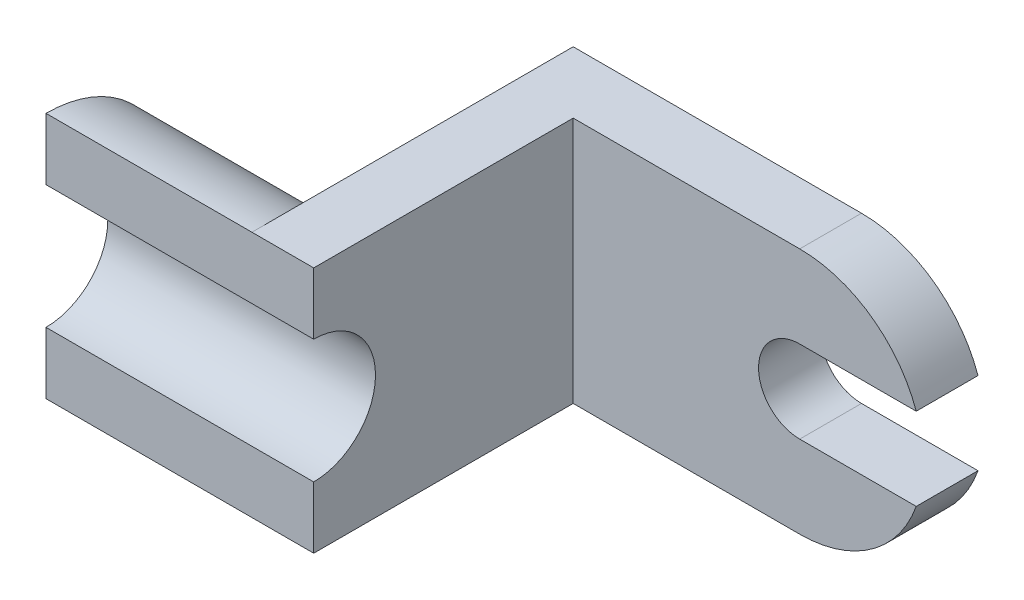
ISO-10303-21;
HEADER;
FILE_DESCRIPTION(('STEP AP214'),'2;1');
FILE_NAME('part.step','',(''),(''),'','','');
FILE_SCHEMA(('AUTOMOTIVE_DESIGN { 1 0 10303 214 1 1 1 1 }'));
ENDSEC;
DATA;
#1=APPLICATION_CONTEXT('core data for automotive mechanical design processes');
#2=APPLICATION_PROTOCOL_DEFINITION('international standard','automotive_design',2000,#1);
#3=PRODUCT_CONTEXT('',#1,'mechanical');
#4=PRODUCT('Part','Part','',(#3));
#5=PRODUCT_RELATED_PRODUCT_CATEGORY('part','',(#4));
#6=PRODUCT_DEFINITION_FORMATION('','',#4);
#7=PRODUCT_DEFINITION_CONTEXT('part definition',#1,'design');
#8=PRODUCT_DEFINITION('design','',#6,#7);
#9=PRODUCT_DEFINITION_SHAPE('','',#8);
#10=(LENGTH_UNIT() NAMED_UNIT(*) SI_UNIT(.MILLI.,.METRE.));
#11=(NAMED_UNIT(*) PLANE_ANGLE_UNIT() SI_UNIT($,.RADIAN.));
#12=(NAMED_UNIT(*) SI_UNIT($,.STERADIAN.) SOLID_ANGLE_UNIT());
#13=UNCERTAINTY_MEASURE_WITH_UNIT(LENGTH_MEASURE(1.E-05),#10,'distance_accuracy_value','');
#14=(GEOMETRIC_REPRESENTATION_CONTEXT(3) GLOBAL_UNCERTAINTY_ASSIGNED_CONTEXT((#13)) GLOBAL_UNIT_ASSIGNED_CONTEXT((#10,
#11,#12)) REPRESENTATION_CONTEXT('',''));
#15=CARTESIAN_POINT('',(0.,0.,0.));
#16=DIRECTION('',(0.,0.,1.));
#17=DIRECTION('',(1.,0.,0.));
#18=AXIS2_PLACEMENT_3D('',#15,#16,#17);
#19=CARTESIAN_POINT('',(15.,60.,78.));
#20=DIRECTION('',(0.,0.,1.));
#21=DIRECTION('',(0.,-1.,0.));
#22=AXIS2_PLACEMENT_3D('',#19,#20,#21);
#23=PLANE('',#22);
#24=DIRECTION('',(0.,1.,0.));
#25=VECTOR('',#24,1.);
#26=CARTESIAN_POINT('',(15.,60.,78.));
#27=LINE('',#26,#25);
#28=CARTESIAN_POINT('',(15.,0.,78.));
#29=VERTEX_POINT('',#28);
#30=CARTESIAN_POINT('',(15.,15.,78.));
#31=VERTEX_POINT('',#30);
#32=EDGE_CURVE('E149',#29,#31,#27,.T.);
#33=ORIENTED_EDGE('',*,*,#32,.T.);
#34=DIRECTION('',(1.,0.,0.));
#35=VECTOR('',#34,1.);
#36=CARTESIAN_POINT('',(-50.,15.,78.));
#37=LINE('',#36,#35);
#38=CARTESIAN_POINT('',(-50.,15.,78.));
#39=VERTEX_POINT('',#38);
#40=EDGE_CURVE('E132',#39,#31,#37,.T.);
#41=ORIENTED_EDGE('',*,*,#40,.F.);
#42=DIRECTION('',(0.,1.,0.));
#43=VECTOR('',#42,1.);
#44=CARTESIAN_POINT('',(-50.,15.,78.));
#45=LINE('',#44,#43);
#46=CARTESIAN_POINT('',(-50.,0.,78.));
#47=VERTEX_POINT('',#46);
#48=EDGE_CURVE('E243',#47,#39,#45,.T.);
#49=ORIENTED_EDGE('',*,*,#48,.F.);
#50=DIRECTION('',(1.,0.,0.));
#51=VECTOR('',#50,1.);
#52=CARTESIAN_POINT('',(-50.,0.,78.));
#53=LINE('',#52,#51);
#54=CARTESIAN_POINT('',(0.,0.,78.));
#55=VERTEX_POINT('',#54);
#56=EDGE_CURVE('E141',#47,#55,#53,.T.);
#57=ORIENTED_EDGE('',*,*,#56,.T.);
#58=DIRECTION('',(-1.,0.,0.));
#59=VECTOR('',#58,1.);
#60=CARTESIAN_POINT('',(15.,0.,78.));
#61=LINE('',#60,#59);
#62=EDGE_CURVE('E160',#29,#55,#61,.T.);
#63=ORIENTED_EDGE('',*,*,#62,.F.);
#64=EDGE_LOOP('',(#33,#41,#49,#57,#63));
#65=FACE_BOUND('',#64,.T.);
#66=ADVANCED_FACE('F39',(#65),#23,.T.);
#67=CARTESIAN_POINT('',(0.,0.,15.));
#68=DIRECTION('',(1.,0.,0.));
#69=DIRECTION('',(0.,0.,-1.));
#70=AXIS2_PLACEMENT_3D('',#67,#68,#69);
#71=PLANE('',#70);
#72=CARTESIAN_POINT('',(0.,30.,78.));
#73=DIRECTION('',(-1.,0.,0.));
#74=DIRECTION('',(0.,0.,1.));
#75=AXIS2_PLACEMENT_3D('',#72,#73,#74);
#76=CIRCLE('',#75,30.);
#77=CARTESIAN_POINT('',(0.,60.,78.));
#78=VERTEX_POINT('',#77);
#79=EDGE_CURVE('E155',#78,#55,#76,.T.);
#80=ORIENTED_EDGE('',*,*,#79,.F.);
#81=DIRECTION('',(0.,0.,-1.));
#82=VECTOR('',#81,1.);
#83=CARTESIAN_POINT('',(0.,60.,15.));
#84=LINE('',#83,#82);
#85=CARTESIAN_POINT('',(0.,60.,0.));
#86=VERTEX_POINT('',#85);
#87=EDGE_CURVE('E220',#78,#86,#84,.T.);
#88=ORIENTED_EDGE('',*,*,#87,.T.);
#89=DIRECTION('',(0.,-1.,0.));
#90=VECTOR('',#89,1.);
#91=CARTESIAN_POINT('',(0.,0.,0.));
#92=LINE('',#91,#90);
#93=CARTESIAN_POINT('',(0.,0.,0.));
#94=VERTEX_POINT('',#93);
#95=EDGE_CURVE('E199',#86,#94,#92,.T.);
#96=ORIENTED_EDGE('',*,*,#95,.T.);
#97=DIRECTION('',(0.,0.,-1.));
#98=VECTOR('',#97,1.);
#99=CARTESIAN_POINT('',(0.,0.,15.));
#100=LINE('',#99,#98);
#101=EDGE_CURVE('E206',#55,#94,#100,.T.);
#102=ORIENTED_EDGE('',*,*,#101,.F.);
#103=EDGE_LOOP('',(#80,#88,#96,#102));
#104=FACE_BOUND('',#103,.T.);
#105=ADVANCED_FACE('F237',(#104),#71,.F.);
#106=CARTESIAN_POINT('',(70.,30.,15.));
#107=DIRECTION('',(0.,0.,-1.));
#108=DIRECTION('',(-1.,0.,0.));
#109=AXIS2_PLACEMENT_3D('',#106,#107,#108);
#110=CYLINDRICAL_SURFACE('',#109,30.);
#111=DIRECTION('',(0.,0.,1.));
#112=VECTOR('',#111,1.);
#113=CARTESIAN_POINT('',(98.2842712474619,40.,0.));
#114=LINE('',#113,#112);
#115=CARTESIAN_POINT('',(98.2842712474619,40.,0.));
#116=VERTEX_POINT('',#115);
#117=CARTESIAN_POINT('',(98.2842712474619,40.,15.));
#118=VERTEX_POINT('',#117);
#119=EDGE_CURVE('E191',#116,#118,#114,.T.);
#120=ORIENTED_EDGE('',*,*,#119,.F.);
#121=CARTESIAN_POINT('',(70.,30.,0.));
#122=DIRECTION('',(0.,0.,1.));
#123=DIRECTION('',(-1.,0.,0.));
#124=AXIS2_PLACEMENT_3D('',#121,#122,#123);
#125=CIRCLE('',#124,30.);
#126=CARTESIAN_POINT('',(70.,60.,0.));
#127=VERTEX_POINT('',#126);
#128=EDGE_CURVE('E208',#116,#127,#125,.T.);
#129=ORIENTED_EDGE('',*,*,#128,.T.);
#130=DIRECTION('',(0.,0.,-1.));
#131=VECTOR('',#130,1.);
#132=CARTESIAN_POINT('',(70.,60.,15.));
#133=LINE('',#132,#131);
#134=CARTESIAN_POINT('',(70.,60.,15.));
#135=VERTEX_POINT('',#134);
#136=EDGE_CURVE('E50',#135,#127,#133,.T.);
#137=ORIENTED_EDGE('',*,*,#136,.F.);
#138=CARTESIAN_POINT('',(70.,30.,15.));
#139=DIRECTION('',(0.,0.,1.));
#140=DIRECTION('',(-1.,0.,0.));
#141=AXIS2_PLACEMENT_3D('',#138,#139,#140);
#142=CIRCLE('',#141,30.);
#143=EDGE_CURVE('E200',#118,#135,#142,.T.);
#144=ORIENTED_EDGE('',*,*,#143,.F.);
#145=EDGE_LOOP('',(#120,#129,#137,#144));
#146=FACE_BOUND('',#145,.T.);
#147=ADVANCED_FACE('F273',(#146),#110,.T.);
#148=CARTESIAN_POINT('',(70.,30.,15.));
#149=DIRECTION('',(0.,0.,-1.));
#150=DIRECTION('',(-1.,0.,0.));
#151=AXIS2_PLACEMENT_3D('',#148,#149,#150);
#152=PLANE('',#151);
#153=DIRECTION('',(-1.,0.,0.));
#154=VECTOR('',#153,1.);
#155=CARTESIAN_POINT('',(0.,60.,15.));
#156=LINE('',#155,#154);
#157=CARTESIAN_POINT('',(15.,60.,15.));
#158=VERTEX_POINT('',#157);
#159=EDGE_CURVE('E204',#135,#158,#156,.T.);
#160=ORIENTED_EDGE('',*,*,#159,.T.);
#161=DIRECTION('',(0.,-1.,0.));
#162=VECTOR('',#161,1.);
#163=CARTESIAN_POINT('',(15.,30.,15.));
#164=LINE('',#163,#162);
#165=CARTESIAN_POINT('',(15.,0.,15.));
#166=VERTEX_POINT('',#165);
#167=EDGE_CURVE('E65',#158,#166,#164,.T.);
#168=ORIENTED_EDGE('',*,*,#167,.T.);
#169=DIRECTION('',(1.,0.,0.));
#170=VECTOR('',#169,1.);
#171=CARTESIAN_POINT('',(70.,0.,15.));
#172=LINE('',#171,#170);
#173=CARTESIAN_POINT('',(70.,0.,15.));
#174=VERTEX_POINT('',#173);
#175=EDGE_CURVE('E197',#166,#174,#172,.T.);
#176=ORIENTED_EDGE('',*,*,#175,.T.);
#177=CARTESIAN_POINT('',(98.2842712474619,20.,15.));
#178=VERTEX_POINT('',#177);
#179=EDGE_CURVE('E203',#174,#178,#142,.T.);
#180=ORIENTED_EDGE('',*,*,#179,.T.);
#181=DIRECTION('',(1.,0.,0.));
#182=VECTOR('',#181,1.);
#183=CARTESIAN_POINT('',(0.,20.,15.));
#184=LINE('',#183,#182);
#185=CARTESIAN_POINT('',(70.,20.,15.));
#186=VERTEX_POINT('',#185);
#187=EDGE_CURVE('E184',#186,#178,#184,.T.);
#188=ORIENTED_EDGE('',*,*,#187,.F.);
#189=CARTESIAN_POINT('',(70.,30.,15.));
#190=DIRECTION('',(0.,0.,1.));
#191=DIRECTION('',(1.,0.,0.));
#192=AXIS2_PLACEMENT_3D('',#189,#190,#191);
#193=CIRCLE('',#192,9.99999999999999);
#194=CARTESIAN_POINT('',(70.,40.,15.));
#195=VERTEX_POINT('',#194);
#196=EDGE_CURVE('E173',#195,#186,#193,.T.);
#197=ORIENTED_EDGE('',*,*,#196,.F.);
#198=DIRECTION('',(1.,0.,0.));
#199=VECTOR('',#198,1.);
#200=CARTESIAN_POINT('',(0.,40.,15.));
#201=LINE('',#200,#199);
#202=EDGE_CURVE('E176',#195,#118,#201,.T.);
#203=ORIENTED_EDGE('',*,*,#202,.T.);
#204=ORIENTED_EDGE('',*,*,#143,.T.);
#205=EDGE_LOOP('',(#160,#168,#176,#180,#188,#197,#203,#204));
#206=FACE_BOUND('',#205,.T.);
#207=ADVANCED_FACE('F299',(#206),#152,.F.);
#208=CARTESIAN_POINT('',(70.,30.,0.));
#209=DIRECTION('',(0.,0.,-1.));
#210=DIRECTION('',(-1.,0.,0.));
#211=AXIS2_PLACEMENT_3D('',#208,#209,#210);
#212=PLANE('',#211);
#213=CARTESIAN_POINT('',(70.,0.,0.));
#214=VERTEX_POINT('',#213);
#215=CARTESIAN_POINT('',(98.2842712474619,20.,0.));
#216=VERTEX_POINT('',#215);
#217=EDGE_CURVE('E207',#214,#216,#125,.T.);
#218=ORIENTED_EDGE('',*,*,#217,.F.);
#219=DIRECTION('',(1.,0.,0.));
#220=VECTOR('',#219,1.);
#221=CARTESIAN_POINT('',(70.,0.,0.));
#222=LINE('',#221,#220);
#223=EDGE_CURVE('E187',#94,#214,#222,.T.);
#224=ORIENTED_EDGE('',*,*,#223,.F.);
#225=ORIENTED_EDGE('',*,*,#95,.F.);
#226=DIRECTION('',(-1.,0.,0.));
#227=VECTOR('',#226,1.);
#228=CARTESIAN_POINT('',(0.,60.,0.));
#229=LINE('',#228,#227);
#230=EDGE_CURVE('E215',#127,#86,#229,.T.);
#231=ORIENTED_EDGE('',*,*,#230,.F.);
#232=ORIENTED_EDGE('',*,*,#128,.F.);
#233=DIRECTION('',(1.,0.,0.));
#234=VECTOR('',#233,1.);
#235=CARTESIAN_POINT('',(0.,40.,0.));
#236=LINE('',#235,#234);
#237=CARTESIAN_POINT('',(70.,40.,0.));
#238=VERTEX_POINT('',#237);
#239=EDGE_CURVE('E178',#238,#116,#236,.T.);
#240=ORIENTED_EDGE('',*,*,#239,.F.);
#241=CARTESIAN_POINT('',(70.,30.,0.));
#242=DIRECTION('',(0.,0.,1.));
#243=DIRECTION('',(1.,0.,0.));
#244=AXIS2_PLACEMENT_3D('',#241,#242,#243);
#245=CIRCLE('',#244,9.99999999999999);
#246=CARTESIAN_POINT('',(70.,20.,0.));
#247=VERTEX_POINT('',#246);
#248=EDGE_CURVE('E175',#238,#247,#245,.T.);
#249=ORIENTED_EDGE('',*,*,#248,.T.);
#250=DIRECTION('',(1.,0.,0.));
#251=VECTOR('',#250,1.);
#252=CARTESIAN_POINT('',(0.,20.,0.));
#253=LINE('',#252,#251);
#254=EDGE_CURVE('E172',#247,#216,#253,.T.);
#255=ORIENTED_EDGE('',*,*,#254,.T.);
#256=EDGE_LOOP('',(#218,#224,#225,#231,#232,#240,#249,#255));
#257=FACE_BOUND('',#256,.T.);
#258=ADVANCED_FACE('F232',(#257),#212,.T.);
#259=CARTESIAN_POINT('',(70.,0.,15.));
#260=DIRECTION('',(0.,1.,0.));
#261=DIRECTION('',(0.,0.,1.));
#262=AXIS2_PLACEMENT_3D('',#259,#260,#261);
#263=PLANE('',#262);
#264=ORIENTED_EDGE('',*,*,#175,.F.);
#265=DIRECTION('',(0.,0.,1.));
#266=VECTOR('',#265,1.);
#267=CARTESIAN_POINT('',(15.,0.,78.));
#268=LINE('',#267,#266);
#269=EDGE_CURVE('E165',#166,#29,#268,.T.);
#270=ORIENTED_EDGE('',*,*,#269,.T.);
#271=ORIENTED_EDGE('',*,*,#62,.T.);
#272=ORIENTED_EDGE('',*,*,#101,.T.);
#273=ORIENTED_EDGE('',*,*,#223,.T.);
#274=DIRECTION('',(0.,0.,-1.));
#275=VECTOR('',#274,1.);
#276=CARTESIAN_POINT('',(70.,0.,15.));
#277=LINE('',#276,#275);
#278=EDGE_CURVE('E11',#174,#214,#277,.T.);
#279=ORIENTED_EDGE('',*,*,#278,.F.);
#280=EDGE_LOOP('',(#264,#270,#271,#272,#273,#279));
#281=FACE_BOUND('',#280,.T.);
#282=ADVANCED_FACE('F41',(#281),#263,.F.);
#283=ORIENTED_EDGE('',*,*,#217,.T.);
#284=DIRECTION('',(0.,0.,1.));
#285=VECTOR('',#284,1.);
#286=CARTESIAN_POINT('',(98.2842712474619,20.,0.));
#287=LINE('',#286,#285);
#288=EDGE_CURVE('E194',#216,#178,#287,.T.);
#289=ORIENTED_EDGE('',*,*,#288,.T.);
#290=ORIENTED_EDGE('',*,*,#179,.F.);
#291=ORIENTED_EDGE('',*,*,#278,.T.);
#292=EDGE_LOOP('',(#283,#289,#290,#291));
#293=FACE_BOUND('',#292,.T.);
#294=ADVANCED_FACE('F303',(#293),#110,.T.);
#295=CARTESIAN_POINT('',(0.,60.,15.));
#296=DIRECTION('',(0.,-1.,0.));
#297=DIRECTION('',(1.,0.,0.));
#298=AXIS2_PLACEMENT_3D('',#295,#296,#297);
#299=PLANE('',#298);
#300=ORIENTED_EDGE('',*,*,#230,.T.);
#301=ORIENTED_EDGE('',*,*,#87,.F.);
#302=DIRECTION('',(-1.,0.,0.));
#303=VECTOR('',#302,1.);
#304=CARTESIAN_POINT('',(15.,60.,78.));
#305=LINE('',#304,#303);
#306=CARTESIAN_POINT('',(15.,60.,78.));
#307=VERTEX_POINT('',#306);
#308=EDGE_CURVE('E167',#307,#78,#305,.T.);
#309=ORIENTED_EDGE('',*,*,#308,.F.);
#310=DIRECTION('',(0.,0.,-1.));
#311=VECTOR('',#310,1.);
#312=CARTESIAN_POINT('',(15.,60.,0.));
#313=LINE('',#312,#311);
#314=EDGE_CURVE('E158',#307,#158,#313,.T.);
#315=ORIENTED_EDGE('',*,*,#314,.T.);
#316=ORIENTED_EDGE('',*,*,#159,.F.);
#317=ORIENTED_EDGE('',*,*,#136,.T.);
#318=EDGE_LOOP('',(#300,#301,#309,#315,#316,#317));
#319=FACE_BOUND('',#318,.T.);
#320=ADVANCED_FACE('F221',(#319),#299,.F.);
#321=CARTESIAN_POINT('',(70.,30.,0.));
#322=DIRECTION('',(0.,0.,1.));
#323=DIRECTION('',(1.,0.,0.));
#324=AXIS2_PLACEMENT_3D('',#321,#322,#323);
#325=CYLINDRICAL_SURFACE('',#324,9.99999999999999);
#326=ORIENTED_EDGE('',*,*,#196,.T.);
#327=DIRECTION('',(0.,0.,1.));
#328=VECTOR('',#327,1.);
#329=CARTESIAN_POINT('',(70.,20.,0.));
#330=LINE('',#329,#328);
#331=EDGE_CURVE('E182',#247,#186,#330,.T.);
#332=ORIENTED_EDGE('',*,*,#331,.F.);
#333=ORIENTED_EDGE('',*,*,#248,.F.);
#334=DIRECTION('',(0.,0.,1.));
#335=VECTOR('',#334,1.);
#336=CARTESIAN_POINT('',(70.,40.,0.));
#337=LINE('',#336,#335);
#338=EDGE_CURVE('E186',#238,#195,#337,.T.);
#339=ORIENTED_EDGE('',*,*,#338,.T.);
#340=EDGE_LOOP('',(#326,#332,#333,#339));
#341=FACE_BOUND('',#340,.T.);
#342=ADVANCED_FACE('F291',(#341),#325,.F.);
#343=CARTESIAN_POINT('',(0.,40.,0.));
#344=DIRECTION('',(0.,-1.,0.));
#345=DIRECTION('',(0.,0.,-1.));
#346=AXIS2_PLACEMENT_3D('',#343,#344,#345);
#347=PLANE('',#346);
#348=ORIENTED_EDGE('',*,*,#202,.F.);
#349=ORIENTED_EDGE('',*,*,#338,.F.);
#350=ORIENTED_EDGE('',*,*,#239,.T.);
#351=ORIENTED_EDGE('',*,*,#119,.T.);
#352=EDGE_LOOP('',(#348,#349,#350,#351));
#353=FACE_BOUND('',#352,.T.);
#354=ADVANCED_FACE('F286',(#353),#347,.T.);
#355=CARTESIAN_POINT('',(0.,20.,0.));
#356=DIRECTION('',(0.,-1.,0.));
#357=DIRECTION('',(0.,0.,-1.));
#358=AXIS2_PLACEMENT_3D('',#355,#356,#357);
#359=PLANE('',#358);
#360=ORIENTED_EDGE('',*,*,#187,.T.);
#361=ORIENTED_EDGE('',*,*,#288,.F.);
#362=ORIENTED_EDGE('',*,*,#254,.F.);
#363=ORIENTED_EDGE('',*,*,#331,.T.);
#364=EDGE_LOOP('',(#360,#361,#362,#363));
#365=FACE_BOUND('',#364,.T.);
#366=ADVANCED_FACE('F285',(#365),#359,.F.);
#367=CARTESIAN_POINT('',(15.,0.,0.));
#368=DIRECTION('',(1.,0.,0.));
#369=DIRECTION('',(0.,0.,-1.));
#370=AXIS2_PLACEMENT_3D('',#367,#368,#369);
#371=PLANE('',#370);
#372=CARTESIAN_POINT('',(15.,30.,78.));
#373=DIRECTION('',(1.,0.,0.));
#374=DIRECTION('',(0.,0.,-1.));
#375=AXIS2_PLACEMENT_3D('',#372,#373,#374);
#376=CIRCLE('',#375,15.);
#377=CARTESIAN_POINT('',(15.,45.,78.));
#378=VERTEX_POINT('',#377);
#379=EDGE_CURVE('E139',#31,#378,#376,.T.);
#380=ORIENTED_EDGE('',*,*,#379,.F.);
#381=ORIENTED_EDGE('',*,*,#32,.F.);
#382=ORIENTED_EDGE('',*,*,#269,.F.);
#383=ORIENTED_EDGE('',*,*,#167,.F.);
#384=ORIENTED_EDGE('',*,*,#314,.F.);
#385=EDGE_CURVE('E151',#378,#307,#27,.T.);
#386=ORIENTED_EDGE('',*,*,#385,.F.);
#387=EDGE_LOOP('',(#380,#381,#382,#383,#384,#386));
#388=FACE_BOUND('',#387,.T.);
#389=ADVANCED_FACE('F150',(#388),#371,.T.);
#390=DIRECTION('',(1.,0.,0.));
#391=VECTOR('',#390,1.);
#392=CARTESIAN_POINT('',(-50.,45.,78.));
#393=LINE('',#392,#391);
#394=CARTESIAN_POINT('',(-50.,45.,78.));
#395=VERTEX_POINT('',#394);
#396=EDGE_CURVE('E53',#395,#378,#393,.T.);
#397=ORIENTED_EDGE('',*,*,#396,.T.);
#398=ORIENTED_EDGE('',*,*,#385,.T.);
#399=ORIENTED_EDGE('',*,*,#308,.T.);
#400=DIRECTION('',(1.,0.,0.));
#401=VECTOR('',#400,1.);
#402=CARTESIAN_POINT('',(-50.,60.,78.));
#403=LINE('',#402,#401);
#404=CARTESIAN_POINT('',(-50.,60.,78.));
#405=VERTEX_POINT('',#404);
#406=EDGE_CURVE('E249',#405,#78,#403,.T.);
#407=ORIENTED_EDGE('',*,*,#406,.F.);
#408=DIRECTION('',(0.,1.,0.));
#409=VECTOR('',#408,1.);
#410=CARTESIAN_POINT('',(-50.,60.,78.));
#411=LINE('',#410,#409);
#412=EDGE_CURVE('E255',#395,#405,#411,.T.);
#413=ORIENTED_EDGE('',*,*,#412,.F.);
#414=EDGE_LOOP('',(#397,#398,#399,#407,#413));
#415=FACE_BOUND('',#414,.T.);
#416=ADVANCED_FACE('F267',(#415),#23,.T.);
#417=CARTESIAN_POINT('',(-50.,30.,78.));
#418=DIRECTION('',(1.,0.,0.));
#419=DIRECTION('',(0.,0.,-1.));
#420=AXIS2_PLACEMENT_3D('',#417,#418,#419);
#421=CYLINDRICAL_SURFACE('',#420,30.);
#422=ORIENTED_EDGE('',*,*,#79,.T.);
#423=ORIENTED_EDGE('',*,*,#56,.F.);
#424=CARTESIAN_POINT('',(-50.,30.,78.));
#425=DIRECTION('',(-1.,0.,0.));
#426=DIRECTION('',(0.,0.,1.));
#427=AXIS2_PLACEMENT_3D('',#424,#425,#426);
#428=CIRCLE('',#427,30.);
#429=EDGE_CURVE('E248',#405,#47,#428,.T.);
#430=ORIENTED_EDGE('',*,*,#429,.F.);
#431=ORIENTED_EDGE('',*,*,#406,.T.);
#432=EDGE_LOOP('',(#422,#423,#430,#431));
#433=FACE_BOUND('',#432,.T.);
#434=ADVANCED_FACE('F246',(#433),#421,.T.);
#435=CARTESIAN_POINT('',(-50.,30.,78.));
#436=DIRECTION('',(1.,0.,0.));
#437=DIRECTION('',(0.,0.,-1.));
#438=AXIS2_PLACEMENT_3D('',#435,#436,#437);
#439=CYLINDRICAL_SURFACE('',#438,15.);
#440=ORIENTED_EDGE('',*,*,#379,.T.);
#441=ORIENTED_EDGE('',*,*,#396,.F.);
#442=CARTESIAN_POINT('',(-50.,30.,78.));
#443=DIRECTION('',(1.,0.,0.));
#444=DIRECTION('',(0.,0.,1.));
#445=AXIS2_PLACEMENT_3D('',#442,#443,#444);
#446=CIRCLE('',#445,15.);
#447=EDGE_CURVE('E140',#39,#395,#446,.T.);
#448=ORIENTED_EDGE('',*,*,#447,.F.);
#449=ORIENTED_EDGE('',*,*,#40,.T.);
#450=EDGE_LOOP('',(#440,#441,#448,#449));
#451=FACE_BOUND('',#450,.T.);
#452=ADVANCED_FACE('F137',(#451),#439,.F.);
#453=CARTESIAN_POINT('',(-50.,30.,78.));
#454=DIRECTION('',(-1.,0.,0.));
#455=DIRECTION('',(0.,0.,1.));
#456=AXIS2_PLACEMENT_3D('',#453,#454,#455);
#457=PLANE('',#456);
#458=ORIENTED_EDGE('',*,*,#429,.T.);
#459=ORIENTED_EDGE('',*,*,#48,.T.);
#460=ORIENTED_EDGE('',*,*,#447,.T.);
#461=ORIENTED_EDGE('',*,*,#412,.T.);
#462=EDGE_LOOP('',(#458,#459,#460,#461));
#463=FACE_BOUND('',#462,.T.);
#464=ADVANCED_FACE('F259',(#463),#457,.T.);
#465=CLOSED_SHELL('',(#66,#105,#147,#207,#258,#282,#294,#320,#342,#354,#366,#389,#416,#434,#452,#464));
#466=MANIFOLD_SOLID_BREP('B2',#465);
#467=ADVANCED_BREP_SHAPE_REPRESENTATION('',(#18,#466),#14);
#468=SHAPE_DEFINITION_REPRESENTATION(#9,#467);
ENDSEC;
END-ISO-10303-21;
